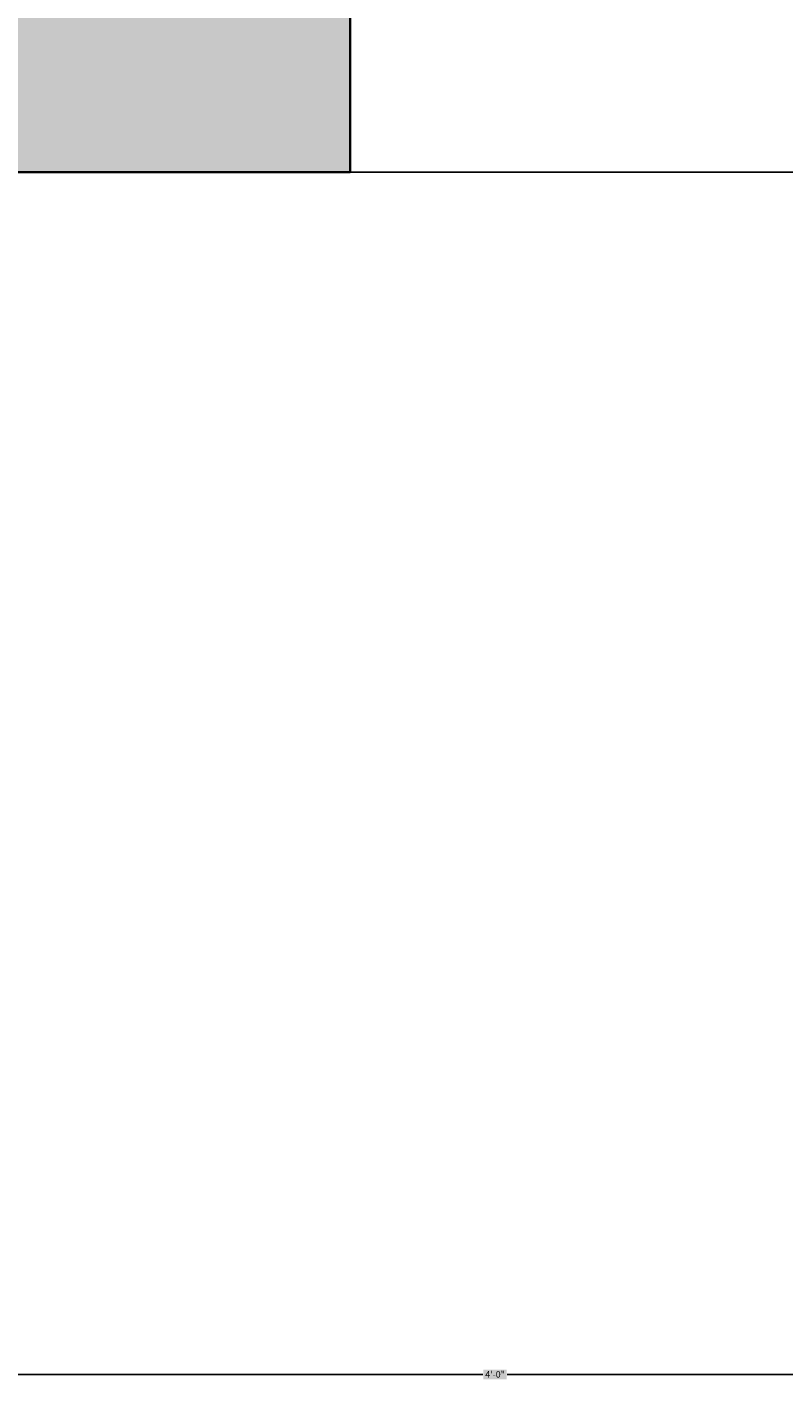
# Model space of a CAD drawing. Units: inches. Extents: x -301 to 715, y -607 to 364.
# Tile 3 of 141: x -24 to -3, y -574 to -536. Entities that reach past the tile are written whole.
import ezdxf

# ---------------------------------------------------------------- set-up
doc = ezdxf.new("R2010")
doc.units = ezdxf.units.IN
doc.header["$MEASUREMENT"] = 0
for name, color, linetype, lineweight in [('A-ANNO-DIMS', 2, 'Continuous', 18), ('A-SECT-PATT', 8, 'Continuous', 13), ('S-FNDN', 2, 'Continuous', 35)]:
    doc.layers.add(name, color=color, linetype=linetype, lineweight=lineweight)
doc.styles.get("Standard").update_dxf_attribs({"font": 'arial.ttf'})
doc.dimstyles.get("Standard").update_dxf_attribs({"dimtxt": 0.18, "dimasz": 0.18, "dimexe": 0.18, "dimexo": 0.0625, "dimgap": 0.09, "dimtad": 0, "dimtih": 1, "dimtoh": 1, "dimdec": 1, "dimzin": 0, "dimdsep": 46, "dimlunit": 4, "dimtxsty": 'Standard', "dimcen": 0.09, "dimclrd": 3, "dimclre": 4, "dimclrt": 6, "dimadec": 0, "dimazin": 0, "dimtfac": 1, "dimtdec": 1, "dimtofl": 0, "dimtmove": 0, "dimatfit": 3, "dimfxl": 1, "dimtfill": 2, "dimtfillclr": 51, "dimtolj": 1, "dimtzin": 0, "dimarcsym": 0})

# ---------------------------------------------------------------- blocks, each defined once
blk = doc.blocks.new('*D176')
at = {"layer": 'A-ANNO-DIMS', "color": 4, "lineweight": -2, "transparency": 16777216}
for p, q in [((148.28, -324.477), (215.605, -324.477)), ((-15.22, -540.477), (215.605, -540.477))]:
    blk.add_line(p, q, dxfattribs=at)
at = {"layer": 'A-ANNO-DIMS', "color": 3, "lineweight": -2, "transparency": 16777216}
for p, q in [((215.425, -324.657), (215.425, -432.296)), ((215.425, -540.297), (215.425, -432.659))]:
    blk.add_line(p, q, dxfattribs=at)
at = {"layer": 'A-ANNO-DIMS', "color": 3, "transparency": 16777216}
for points in [[(215.395, -324.657), (215.455, -324.657), (215.425, -324.477)], [(215.395, -540.297), (215.455, -540.297), (215.425, -540.477)]]:
    blk.add_solid(points, dxfattribs=at)
at = {"layer": 'Defpoints', "color": 0, "transparency": 16777216}
for p in [(148.218, -324.477), (-15.282, -540.477), (215.425, -540.477)]:
    blk.add_point(p, dxfattribs=at)
at = {"layer": 'A-ANNO-DIMS', "color": 6, "transparency": 16777216, "insert": (215.425, -432.477), "char_height": 0.18, "attachment_point": 5, "bg_fill": 1, "box_fill_scale": 1.25, "bg_fill_color": 51, "bg_fill_transparency": 0}
blk.add_mtext('\\A1;18\'-0"', dxfattribs=at)
blk = doc.blocks.new('*D180')
at = {"layer": 'A-ANNO-DIMS', "color": 4, "lineweight": -2, "transparency": 16777216}
for p, q in [((-35.282, -463.54), (-35.282, -573.809)), ((12.718, -463.54), (12.718, -573.809))]:
    blk.add_line(p, q, dxfattribs=at)
at = {"layer": 'A-ANNO-DIMS', "color": 3, "lineweight": -2, "transparency": 16777216}
for p, q in [((-35.102, -573.629), (-11.615, -573.629)), ((12.538, -573.629), (-10.949, -573.629))]:
    blk.add_line(p, q, dxfattribs=at)
at = {"layer": 'A-ANNO-DIMS', "color": 3, "transparency": 16777216}
for points in [[(-35.102, -573.599), (-35.102, -573.659), (-35.282, -573.629)], [(12.538, -573.599), (12.538, -573.659), (12.718, -573.629)]]:
    blk.add_solid(points, dxfattribs=at)
at = {"layer": 'Defpoints', "color": 0, "transparency": 16777216}
for p in [(-35.282, -463.477), (12.718, -463.477), (12.718, -573.629)]:
    blk.add_point(p, dxfattribs=at)
at = {"layer": 'A-ANNO-DIMS', "color": 6, "transparency": 16777216, "insert": (-11.282, -573.629), "char_height": 0.18, "attachment_point": 5, "bg_fill": 1, "box_fill_scale": 1.25, "bg_fill_color": 51, "bg_fill_transparency": 0}
blk.add_mtext('\\A1;4\'-0"', dxfattribs=at)
blk = doc.blocks.new('*D191')
at = {"layer": 'A-ANNO-DIMS', "color": 4, "lineweight": -2, "transparency": 16777216}
for p, q in [((129.193, -481.477), (-266.112, -481.477)), ((114.193, -540.477), (-266.112, -540.477))]:
    blk.add_line(p, q, dxfattribs=at)
at = {"layer": 'A-ANNO-DIMS', "color": 3, "lineweight": -2, "transparency": 16777216}
for p, q in [((-265.932, -481.657), (-265.932, -510.797)), ((-265.932, -540.297), (-265.932, -511.158))]:
    blk.add_line(p, q, dxfattribs=at)
at = {"layer": 'A-ANNO-DIMS', "color": 3, "transparency": 16777216}
for points in [[(-265.962, -481.657), (-265.902, -481.657), (-265.932, -481.477)], [(-265.962, -540.297), (-265.902, -540.297), (-265.932, -540.477)]]:
    blk.add_solid(points, dxfattribs=at)
at = {"layer": 'Defpoints', "color": 0, "transparency": 16777216}
for p in [(129.255, -481.477), (-265.932, -540.477), (114.255, -540.477)]:
    blk.add_point(p, dxfattribs=at)
at = {"layer": 'A-ANNO-DIMS', "color": 6, "transparency": 16777216, "insert": (-265.932, -510.977), "char_height": 0.18, "attachment_point": 5, "bg_fill": 1, "box_fill_scale": 1.25, "bg_fill_color": 51, "bg_fill_transparency": 0}
blk.add_mtext('\\A1;4\'-11"', dxfattribs=at)

msp = doc.modelspace()

# ---------------------------------------------------------------- hatches: boundary and pattern name
at = {"layer": 'A-SECT-PATT'}
h = msp.add_hatch(dxfattribs=at)
h.set_pattern_fill('AR-CONC', color=256, scale=0.5)
h.set_pattern_definition([(50, (10.3213, 33.8764), (3.586301, -0.31376), [0.375, -4.125]), (355, (10.3213, 33.8764), (-0.693757, 3.76096), [0.3, -3.3]), (100.45144, (10.62, 33.8502), (2.892544, 3.4472), [0.3187, -3.50571]), (46.1842, (10.3213, 34.8764), (5.336207, -0.827596), [0.5625, -6.1875]), (96.6356, (10.766, 34.8074), (4.67331, 4.870593), [0.47805, -5.25857]), (351.1842, (10.321, 34.8764), (4.67331, 4.870593), [0.45, -4.95]), (21, (10.8213, 34.6264), (2.984535, -2.013094), [0.375, -4.125]), (326, (10.8213, 34.6264), (1.216577, 3.62575), [0.3, -3.3]), (71.45144, (11.07, 34.4586), (4.201112, 1.612656), [0.3187, -3.50571]), (37.5, (10.3213, 33.8764), (0.0607993, 1.6644693), [0, -3.26, 0, -3.35, 0, -3.3125]), (7.5, (10.3213, 33.8764), (1.3153477, 1.9720586), [0, -1.91, 0, -3.185, 0, -1.2625]), (327.5, (9.2063, 33.8764), (2.6691122, -0.1127744), [0, -1.25, 0, -3.9, 0, -5.175]), (317.5, (8.7063, 33.8764), (2.915931, 0.500525), [0, -1.625, 0, -2.59, 0, -3.675])])
h.paths.add_polyline_path([(-56.282, -535.477), (-61.282, -535.477), (-61.282, -540.477), (-15.282, -540.477), (-15.282, -535.477), (-20.282, -535.477)])
h.paths.add_polyline_path([(119.255, -535.477), (114.255, -535.477), (114.255, -540.477), (163.255, -540.477), (163.255, -535.477), (158.255, -535.477)])
h.paths.add_polyline_path([(-206.282, -471.477), (-209.282, -471.477), (-209.282, -481.477), (-206.282, -481.477), (-194.282, -481.477), (-194.282, -471.477)])
h.paths.add_polyline_path([(-41.282, -481.477), (-41.282, -471.477), (-185.282, -471.477), (-185.282, -481.477), (-180.282, -481.477)])
h.paths.add_polyline_path([(134.255, -481.477), (134.255, -471.477), (-35.282, -471.477), (-35.282, -481.477), (-30.282, -481.477)])
h.paths.add_polyline_path([(155.218, -481.477), (158.218, -481.477), (158.218, -471.477), (153.218, -471.477), (143.218, -471.477), (143.218, -481.477), (148.255, -481.477)])
h.paths.add_polyline_path([(-193.88, -356.477), (-193.904, -361.477), (143.218, -361.477), (143.218, -356.477)])

# ---------------------------------------------------------------- linework, layer by layer
at = {"layer": 'S-FNDN'}
for p in [(-15.282, -535.477), (-61.282, -540.477)]:
    msp.add_line(p, (-15.282, -540.477), dxfattribs=at)

# ---------------------------------------------------------------- dimensions: what is measured, and where the dimension line sits
at = {"layer": 'A-ANNO-DIMS'}
for base, p1, p2, picture, middle in [((215.425, -540.477), (148.218, -324.477), (-15.282, -540.477), '*D176', (215.425, -432.477)), ((-265.932, -540.477), (129.255, -481.477), (114.255, -540.477), '*D191', (-265.932, -510.977))]:
    dim = msp.add_linear_dim(base=base, p1=p1, p2=p2, angle=90, dimstyle='Standard', override={"dimdec": 1, "dimlfac": 1, "dimrnd": 0, "dimzin": 1, "dimdsep": 46, "dimlunit": 4, "dimfrac": 2}, dxfattribs=at)
    dim.commit()
    dim.dimension.update_dxf_attribs({"geometry": picture, "text_midpoint": middle})
dim = msp.add_linear_dim(base=(12.718, -573.629), p1=(-35.282, -463.477), p2=(12.718, -463.477), dimstyle='Standard', override={"dimdec": 1, "dimlfac": 1, "dimrnd": 0, "dimzin": 1, "dimdsep": 46, "dimlunit": 4, "dimfrac": 2}, dxfattribs=at)
dim.commit()
dim.dimension.update_dxf_attribs({"geometry": '*D180', "text_midpoint": (-11.282, -573.629)})

doc.saveas('drawing.dxf')
